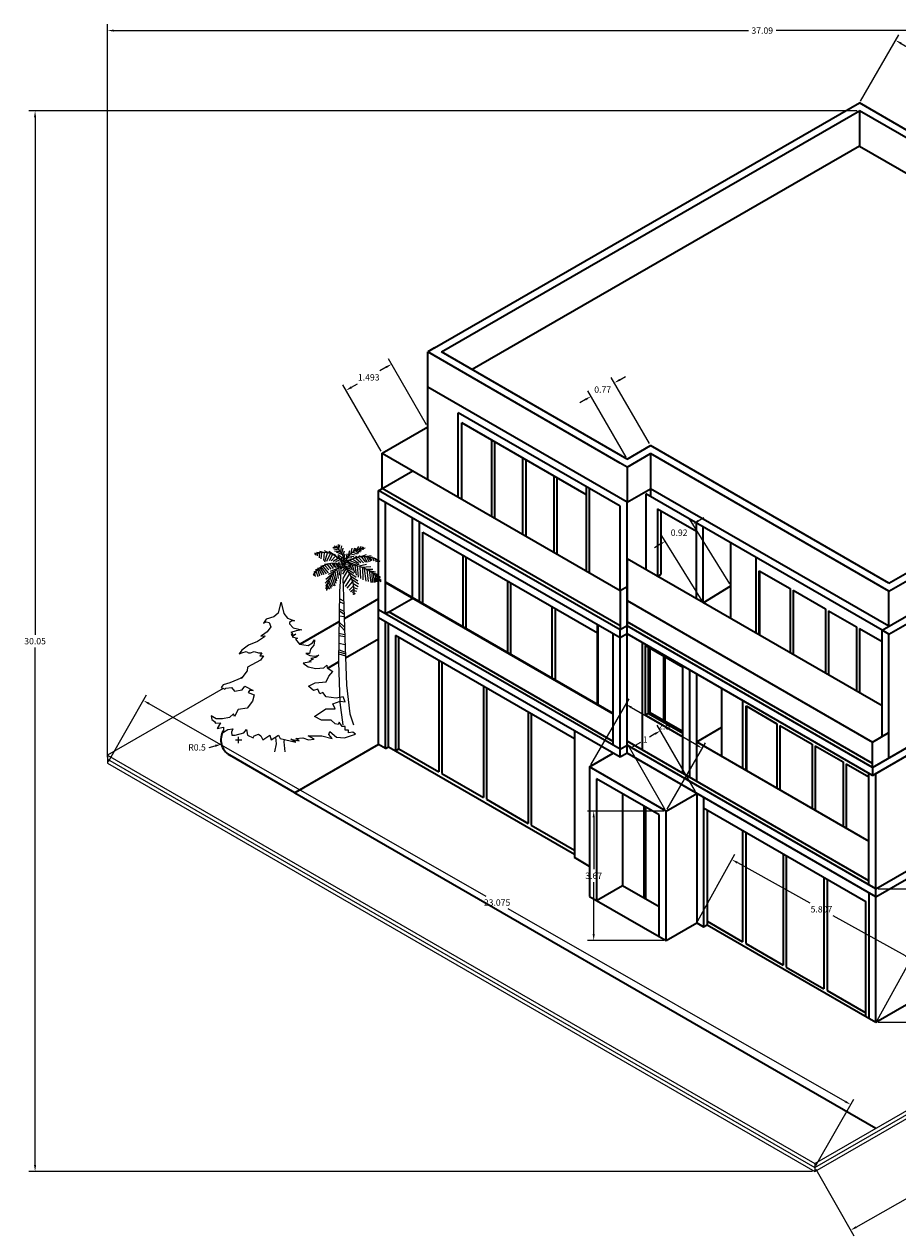
# Model space of a CAD drawing. Units: metres. Extents: x 5057 to 10150, y 1364 to 2760.
# Tile 1 of 2: x 5057 to 5082, y 1364 to 1399. Entities that reach past the tile are written whole.
import ezdxf

# ---------------------------------------------------------------- set-up
doc = ezdxf.new("R2010")
doc.units = ezdxf.units.M
for name, color, linetype, lineweight in [('A-ANNO-DIMS', 2, 'Continuous', 18), ('A-ANNO-NPLT', 8, 'Continuous', 13), ('A-ELEV', 7, 'Continuous', 35), ('C-SITE', 3, 'Continuous', 25), ('L-PLNT', 3, 'Continuous', 13)]:
    doc.layers.add(name, color=color, linetype=linetype, lineweight=lineweight)
doc.styles.get("Standard").update_dxf_attribs({"font": 'arial.ttf'})
doc.dimstyles.get("Standard").update_dxf_attribs({"dimtxt": 0.18, "dimasz": 0.18, "dimexe": 0.18, "dimexo": 0.0625, "dimgap": 0.09, "dimtad": 0, "dimtih": 1, "dimtoh": 1, "dimdec": 4, "dimzin": 0, "dimdsep": 46, "dimtxsty": 'Standard', "dimcen": 0.09, "dimadec": 0, "dimazin": 0, "dimtfac": 1, "dimtdec": 4, "dimtofl": 0, "dimtmove": 0, "dimatfit": 3, "dimfxl": 1, "dimtolj": 1, "dimtzin": 0, "dimarcsym": 0})

# ---------------------------------------------------------------- blocks, each defined once
blk = doc.blocks.new('*U3')
for p, q in [((-29.729, 190.759), (-31.469, 191.255)), ((-30.309, 190.512), (-30.695, 189.025)), ((-25.283, 191.751), (-29.342, 192.246)), ((-28.763, 190.759), (-28.763, 188.281)), ((-26.443, 191.503), (-26.636, 186.051)), ((-20.064, 191.751), (-25.863, 193.238)), ((-23.737, 191.751), (-24.51, 185.06)), ((-21.031, 191.998), (-21.804, 183.325)), ((-15.232, 191.255), (-20.644, 193.981)), ((-17.551, 191.503), (-20.451, 181.343)), ((-14.265, 190.759), (-18.131, 182.086)), ((-9.433, 189.025), (-15.618, 193.238)), ((-11.753, 189.768), (-15.425, 182.83)), ((-6.727, 197.202), (-11.366, 197.45)), ((-3.441, 194.477), (-10.013, 195.716)), ((-1.894, 192.494), (-9.24, 193.733)), ((-6.147, 186.299), (-9.24, 190.264)), ((-7.5, 199.68), (-7.5, 197.946)), ((-0.541, 189.52), (-7.307, 192.494)), ((-5.76, 190.016), (0.618, 185.308)), ((-5.567, 196.707), (-4.987, 201.167)), ((-4.407, 195.716), (-3.247, 200.672)), ((-2.474, 193.733), (-1.315, 199.433)), ((-1.121, 190.759), (0.232, 196.955)), ((0.038, 188.281), (1.778, 193.981)), ((1.005, 185.803), (2.358, 190.759)), ((4.098, 185.06), (4.678, 190.512)), ((5.837, 187.786), (7.577, 194.229)), ((8.544, 190.512), (13.763, 189.52)), ((9.317, 191.255), (10.283, 196.955)), ((11.25, 192.494), (15.889, 190.512)), ((11.829, 192.99), (13.182, 197.45)), ((13.956, 194.229), (14.729, 196.955)), ((14.536, 193.981), (17.242, 191.255)), ((15.116, 194.477), (17.822, 198.689)), ((16.082, 194.972), (17.822, 192.494)), ((18.015, 195.716), (20.914, 198.689)), ((18.015, 195.468), (18.981, 192.494)), ((19.368, 196.459), (19.948, 193.733)), ((19.368, 187.29), (26.133, 189.768)), ((20.914, 196.459), (21.301, 194.972)), ((21.301, 196.459), (22.847, 198.441)), ((22.074, 196.707), (23.427, 195.716)), ((23.234, 196.707), (23.62, 197.698)), ((-21.031, 177.626), (-24.897, 176.387)), ((-24.317, 175.891), (-18.711, 168.457)), ((-22.191, 176.635), (-16.391, 169.448)), ((-15.618, 179.36), (-20.644, 178.617)), ((-20.064, 177.626), (-15.812, 172.67)), ((-17.358, 178.617), (-13.299, 173.661)), ((-15.038, 179.36), (-10.786, 174.404)), ((-8.08, 188.034), (-12.912, 182.83)), ((-12.332, 180.104), (-9.433, 175.643)), ((-4.987, 185.803), (-10.979, 182.086)), ((-10.206, 180.104), (-8.08, 175.891)), ((-1.701, 176.882), (-8.66, 175.396)), ((-8.273, 180.104), (-6.147, 176.635)), ((-3.247, 183.821), (-8.08, 181.838)), ((-6.34, 179.608), (-4.6, 177.13)), ((-5.76, 188.034), (-1.508, 182.582)), ((-1.315, 181.591), (-5.374, 181.095)), ((-4.021, 179.36), (-2.861, 177.378)), ((-2.668, 185.803), (1.198, 181.343)), ((-2.668, 176.387), (-2.376, 170.594)), ((-0.348, 180.352), (-1.894, 180.104)), ((-0.928, 176.882), (-1.508, 173.909)), ((2.551, 175.891), (-0.928, 171.431)), ((1.585, 177.13), (0.038, 174.652)), ((1.005, 182.582), (2.938, 186.547)), ((1.585, 177.13), (6.61, 176.139)), ((2.938, 182.582), (6.61, 183.821)), ((2.938, 175.891), (8.737, 173.413)), ((4.098, 180.847), (8.35, 179.608)), ((4.871, 186.051), (10.09, 186.547)), ((4.871, 181.591), (8.544, 184.812)), ((5.644, 181.838), (13.569, 178.865)), ((6.224, 178.121), (8.157, 175.148)), ((6.997, 188.529), (12.216, 187.786)), ((7.384, 178.369), (10.476, 179.36)), ((7.77, 183.325), (16.082, 179.856)), ((8.157, 178.121), (10.476, 172.422)), ((9.51, 184.317), (15.502, 188.034)), ((10.476, 177.874), (12.796, 169.696)), ((11.25, 184.812), (17.628, 180.352)), ((11.829, 177.874), (18.015, 179.113)), ((13.182, 177.874), (14.729, 166.97)), ((14.536, 185.803), (19.948, 180.847)), ((15.695, 186.299), (19.368, 188.777)), ((15.889, 177.13), (16.855, 164.492)), ((17.242, 186.547), (23.041, 180.599)), ((18.015, 177.13), (26.133, 179.113)), ((18.981, 175.891), (19.561, 163.005)), ((20.721, 187.042), (25.167, 181.343)), ((20.914, 175.891), (30.966, 176.635)), ((23.814, 187.29), (26.907, 181.343)), ((24.78, 187.538), (31.546, 188.777)), ((26.133, 187.29), (29.419, 181.838)), ((28.066, 187.29), (30.966, 182.582)), ((29.806, 186.795), (32.319, 183.078)), ((29.999, 186.795), (33.092, 187.29)), ((32.512, 186.299), (35.218, 186.299)), ((33.479, 186.051), (34.445, 182.83)), ((35.605, 185.556), (37.151, 185.308)), ((35.798, 185.308), (36.958, 181.591)), ((38.118, 184.317), (38.504, 181.838)), ((39.857, 182.83), (40.244, 181.591)), ((-32.628, 167.961), (-33.208, 167.961)), ((-32.628, 167.713), (-32.435, 165.979)), ((-28.956, 172.174), (-32.435, 170.192)), ((-31.082, 169.944), (-32.435, 169.2)), ((-31.662, 168.705), (-31.082, 165.483)), ((-27.409, 173.413), (-30.695, 172.67)), ((-29.922, 170.687), (-27.989, 165.235)), ((-25.09, 175.148), (-28.376, 174.404)), ((-27.989, 172.422), (-26.056, 166.227)), ((-26.829, 173.661), (-23.544, 167.218)), ((-25.476, 174.652), (-21.224, 167.466)), ((-14.265, 164.244), (-19.678, 158.049)), ((-12.139, 167.961), (-19.098, 162.014)), ((-8.466, 171.678), (-16.585, 167.713)), ((-14.265, 163.749), (-10.786, 154.828)), ((-4.214, 175.148), (-14.072, 170.935)), ((-12.719, 166.722), (-9.046, 154.828)), ((-10.979, 168.457), (-7.887, 157.801)), ((-8.853, 170.935), (-7.113, 160.527)), ((-6.92, 172.917), (-5.374, 163.253)), ((-4.6, 174.9), (-4.021, 166.722)), ((3.711, 174.404), (-0.541, 167.961)), ((5.257, 171.926), (-0.155, 163.005)), ((7.384, 168.705), (0.812, 157.553)), ((9.317, 164.244), (2.358, 154.332)), ((4.291, 173.909), (12.216, 168.953)), ((6.417, 170.439), (14.729, 164.492)), ((8.544, 165.979), (16.662, 160.527)), ((10.09, 162.51), (17.435, 157.058)), ((21.688, 175.396), (22.074, 161.518)), ((23.814, 174.404), (25.554, 160.279)), ((25.554, 173.661), (33.285, 173.661)), ((26.52, 173.165), (28.066, 159.784)), ((28.839, 172.174), (36.378, 170.687)), ((29.226, 171.926), (30.966, 158.545)), ((30.966, 170.687), (38.891, 167.713)), ((32.126, 169.696), (32.512, 158.545)), ((34.058, 168.705), (34.445, 158.545)), ((35.412, 167.713), (41.404, 164.988)), ((36.378, 166.474), (35.605, 158.792)), ((37.731, 165.235), (36.958, 159.288)), ((37.924, 165.235), (41.404, 163.749)), ((38.504, 164.492), (38.504, 159.536)), ((39.664, 163.253), (42.37, 161.766)), ((39.857, 162.757), (39.857, 160.031)), ((-16.005, 160.031), (-19.484, 154.084)), ((-18.131, 153.589), (-19.484, 151.606)), ((-17.938, 152.597), (-16.972, 151.111)), ((-17.358, 155.819), (-14.845, 151.358)), ((-16.585, 158.545), (-13.106, 152.35)), ((-15.618, 160.775), (-12.332, 154.332)), ((10.863, 159.784), (4.484, 152.35)), ((11.829, 155.075), (6.804, 150.119)), ((12.603, 151.111), (8.544, 148.385)), ((11.443, 157.553), (16.855, 154.332)), ((12.216, 153.093), (16.082, 151.606)), ((12.603, 149.872), (15.116, 149.128)), ((40.824, 161.766), (41.21, 160.031)), ((41.21, 161.518), (42.757, 160.279)), ((-4.081, 140.645), (0.753, 138.261)), ((-4.081, 137.547), (0.753, 135.163)), ((12.216, 148.137), (10.09, 147.393)), ((12.409, 145.659), (11.056, 145.659)), ((12.409, 146.898), (13.763, 146.402)), ((-4.081, 129.205), (1.124, 126.821)), ((-4.081, 127.298), (1.31, 123.246)), ((-4.453, 112.283), (1.682, 105.133)), ((-4.267, 114.428), (1.682, 108.708)), ((-4.081, 121.578), (1.31, 120.863)), ((-4.639, 102.273), (1.868, 100.604)), ((-4.453, 99.651), (2.24, 98.459)), ((-4.825, 83.921), (2.612, 81.061)), ((-4.639, 81.299), (2.797, 78.916)), ((-4.453, 91.071), (2.426, 89.641)), ((-4.639, 78.916), (2.797, 76.771))]:
    blk.add_line(p, q)
for points in [[(-2.363, 170.553), (-3.88, 148.505), (-4.988, 69.634), (-3.325, 24.869), (0, 0)], [(-0.116, 162.848), (0.554, 143.532), (2.217, 96.635), (3.88, 44.054), (7.76, 12.079), (11.64, 0)]]:
    blk.add_lwpolyline(points)
for centre, radius, start, end in [((-21.738, 166.094), 25.899, 27.67115, 112.5305), ((-18.427, 181.448), 19.715, 350.285, 64.11229), ((25.595, 171.567), 25.395, 91.40319, 163.882), ((-9.259, 151.732), 28.386, 68.38311, 147.5322), ((14.394, 148.393), 32.752, 113.7592, 177.4133), ((23.687, 155.341), 32.188, 56.19272, 134.3213), ((5.828, 132.718), 45.639, 35.98777, 95.82273), ((-32.8, 147.923), 45.309, 356.1943, 41.37848)]:
    blk.add_arc(centre, radius, start, end)
blk = doc.blocks.new('*U5')
for p, q in [((-8.263, 7.598), (-8.747, 14.105)), ((-0.771, 9.56), (-0.69, 11.833)), ((-9.75, 0), (-8.263, 7.598)), ((0, 0), (-0.771, 9.56))]:
    blk.add_line(p, q)
for points in [[(-3.9, 142.35), (-6.596, 132.037), (-10.801, 128.443), (-17.81, 126.047), (-20.614, 122.452), (-17.81, 123.65), (-15.007, 123.051), (-13.605, 118.858), (-16.876, 114.065), (-21.549, 111.07), (-22.951, 109.872), (-19.212, 110.471), (-19.68, 109.273), (-26.222, 105.079), (-34.633, 101.485), (-41.175, 96.693), (-43.511, 93.098), (-41.175, 94.296), (-36.969, 95.494), (-34.633, 94.296), (-32.764, 94.296), (-29.493, 95.494)], [(-3.759, 141.97), (-1.074, 131.643), (2.437, 127.141), (8.84, 124.493), (6.568, 124.493), (4.09, 123.169), (4.296, 121.846), (7.807, 117.874), (16.069, 116.02), (10.492, 115.226), (5.535, 113.372), (6.981, 112.843), (5.948, 110.989), (10.286, 112.048), (6.775, 109.401), (11.732, 108.077), (9.873, 107.282), (13.797, 102.516), (21.852, 101.192), (25.983, 103.84), (28.048, 106.488), (27.842, 105.164), (27.429, 101.457), (24.124, 97.75), (23.091, 93.513), (19.58, 93.513), (23.505, 91.66), (28.255, 90.866), (31.973, 91.925), (29.081, 89.806), (24.537, 88.747), (26.809, 88.218), (22.472, 86.099), (24.95, 85.57), (17.308, 84.246), (21.852, 80.804), (29.081, 79.215), (36.723, 80.009), (39.821, 82.392), (40.028, 80.009), (45.398, 76.567)], [(-29.25, 95.55), (-25.287, 94.296), (-22.016, 94.296), (-23.885, 91.301), (-20.614, 91.301), (-23.418, 87.108), (-35.567, 80.518), (-36.035, 76.924), (-41.175, 70.334), (-52.389, 65.542), (-58.931, 63.744), (-60.8, 61.348), (-57.062, 59.551), (-56.128, 60.749), (-50.987, 61.348), (-48.184, 57.754), (-40.707, 58.952), (-38.371, 62.546), (-30.427, 58.353), (-33.698, 58.353), (-35.1, 56.556), (-29.493, 54.159), (-30.894, 48.169), (-36.035, 41.579), (-44.446, 40.381), (-48.184, 33.791), (-49.118, 36.188), (-52.857, 32.593), (-59.399, 31.395), (-65.473, 31.395), (-70.146, 34.39), (-69.679, 30.796), (-66.875, 28.999), (-65.941, 27.202), (-61.268, 27.801), (-64.539, 22.409), (-58.464, 23.607), (-58.464, 18.815), (-54.258, 21.211), (-49.586, 21.81), (-50.987, 18.815), (-50.52, 15.82), (-47.249, 15.82), (-39.306, 18.216), (-36.502, 21.211), (-35.567, 15.82), (-30.427, 13.423), (-29.493, 15.221), (-25.287, 17.018), (-22.951, 15.221), (-21.081, 11.626), (-14.539, 15.82), (-13.138, 11.626), (-6.128, 15.82), (-4.726, 12.824), (10.226, 9.23), (5.554, 12.225), (13.497, 10.428), (10.226, 12.824), (16.768, 13.423), (22.376, 11.626), (27.516, 12.225), (21.909, 15.221), (34.993, 15.221), (44.806, 12.824), (41.535, 16.419), (42.469, 19.414), (49.011, 14.023), (56.487, 13.423), (66.768, 17.018), (64.431, 18.815), (60.226, 18.216), (60.226, 20.612), (56.955, 20.612), (56.955, 24.206), (54.151, 24.206), (51.348, 28.4), (50.413, 26.004), (47.609, 26.603), (43.871, 30.197), (38.731, 30.197), (34.525, 30.197), (27.983, 33.791), (38.731, 40.98), (47.609, 40.98), (45.273, 45.773), (52.282, 48.169), (56.955, 47.57), (55.086, 52.362), (48.544, 51.164), (39.198, 52.362), (35.927, 56.556), (33.123, 55.357), (31.254, 59.551), (27.049, 58.353), (22.376, 62.546), (28.451, 65.542), (39.198, 66.74), (41.535, 72.131), (45.273, 76.325)]]:
    blk.add_lwpolyline(points)
blk = doc.blocks.new('*D9')
at = {"layer": 'A-ANNO-DIMS', "color": 0, "lineweight": -2, "transparency": 16777216}
for p, q in [((5059.194, 1377.756), (5059.194, 1398.523)), ((5059.374, 1398.343), (5077.345, 1398.343)), ((5096.103, 1398.343), (5078.132, 1398.343)), ((5096.283, 1375.925), (5096.283, 1398.523))]:
    blk.add_line(p, q, dxfattribs=at)
at = {"layer": 'A-ANNO-DIMS', "color": 0, "transparency": 16777216}
for points in [[(5059.374, 1398.373), (5059.374, 1398.313), (5059.194, 1398.343)], [(5096.103, 1398.373), (5096.103, 1398.313), (5096.283, 1398.343)]]:
    blk.add_solid(points, dxfattribs=at)
at = {"layer": 'Defpoints', "color": 0, "transparency": 16777216}
for p in [(5096.283, 1398.343), (5059.194, 1377.694), (5096.283, 1375.863)]:
    blk.add_point(p, dxfattribs=at)
at = {"layer": 'A-ANNO-DIMS', "color": 0, "transparency": 16777216, "insert": (5077.738, 1398.343), "char_height": 0.18, "attachment_point": 5}
blk.add_mtext('\\A1;37.09', dxfattribs=at)
blk = doc.blocks.new('*D10')
at = {"layer": 'A-ANNO-DIMS', "color": 0, "lineweight": -2, "transparency": 16777216}
for p, q in [((5080.427, 1396.067), (5056.964, 1396.067)), ((5057.144, 1395.887), (5057.144, 1381.223)), ((5057.144, 1366.195), (5057.144, 1380.859)), ((5079.164, 1366.015), (5056.964, 1366.015))]:
    blk.add_line(p, q, dxfattribs=at)
at = {"layer": 'A-ANNO-DIMS', "color": 0, "transparency": 16777216}
for points in [[(5057.114, 1395.887), (5057.174, 1395.887), (5057.144, 1396.067)], [(5057.114, 1366.195), (5057.174, 1366.195), (5057.144, 1366.015)]]:
    blk.add_solid(points, dxfattribs=at)
at = {"layer": 'Defpoints', "color": 0, "transparency": 16777216}
for p in [(5057.144, 1396.067), (5080.489, 1396.067), (5079.226, 1366.015)]:
    blk.add_point(p, dxfattribs=at)
at = {"layer": 'A-ANNO-DIMS', "color": 0, "transparency": 16777216, "insert": (5057.144, 1381.041), "char_height": 0.18, "attachment_point": 5}
blk.add_mtext('\\A1;30.05', dxfattribs=at)
blk = doc.blocks.new('*D11')
at = {"layer": 'A-ANNO-DIMS', "color": 0, "lineweight": -2, "transparency": 16777216}
for p, q in [((5059.225, 1377.635), (5060.301, 1379.517)), ((5060.368, 1379.271), (5069.909, 1373.816)), ((5080.088, 1367.997), (5070.546, 1373.452)), ((5079.257, 1366.182), (5080.333, 1368.064))]:
    blk.add_line(p, q, dxfattribs=at)
at = {"layer": 'A-ANNO-DIMS', "color": 0, "transparency": 16777216}
for points in [[(5060.383, 1379.297), (5060.353, 1379.245), (5060.211, 1379.36)], [(5080.102, 1368.023), (5080.073, 1367.971), (5080.244, 1367.908)]]:
    blk.add_solid(points, dxfattribs=at)
at = {"layer": 'Defpoints', "color": 0, "transparency": 16777216}
for p in [(5059.194, 1377.581), (5080.244, 1367.908), (5079.226, 1366.128)]:
    blk.add_point(p, dxfattribs=at)
at = {"layer": 'A-ANNO-DIMS', "color": 0, "transparency": 16777216, "insert": (5070.228, 1373.634), "char_height": 0.18, "attachment_point": 5}
blk.add_mtext('\\A1;23.075', dxfattribs=at)
blk = doc.blocks.new('*D12')
at = {"layer": 'A-ANNO-DIMS', "color": 0, "lineweight": -2, "transparency": 16777216}
for p, q in [((5096.314, 1375.808), (5097.388, 1373.926)), ((5097.143, 1373.993), (5089.09, 1369.397)), ((5080.399, 1364.437), (5088.452, 1369.033)), ((5079.257, 1366.074), (5080.332, 1364.191))]:
    blk.add_line(p, q, dxfattribs=at)
at = {"layer": 'A-ANNO-DIMS', "color": 0, "transparency": 16777216}
for points in [[(5097.128, 1374.019), (5097.158, 1373.967), (5097.299, 1374.082)], [(5080.384, 1364.463), (5080.414, 1364.411), (5080.243, 1364.348)]]:
    blk.add_solid(points, dxfattribs=at)
at = {"layer": 'Defpoints', "color": 0, "transparency": 16777216}
for p in [(5096.283, 1375.863), (5079.226, 1366.128), (5080.243, 1364.348)]:
    blk.add_point(p, dxfattribs=at)
at = {"layer": 'A-ANNO-DIMS', "color": 0, "transparency": 16777216, "insert": (5088.771, 1369.215), "char_height": 0.18, "attachment_point": 5}
blk.add_mtext('\\A1;19.64', dxfattribs=at)
blk = doc.blocks.new('*D17')
at = {"layer": 'A-ANNO-DIMS', "color": 0, "lineweight": -2, "transparency": 16777216}
for p, q in [((5080.521, 1396.347), (5081.604, 1398.224)), ((5081.67, 1397.979), (5084.681, 1396.24)), ((5088.323, 1394.138), (5085.312, 1395.876)), ((5087.485, 1392.327), (5088.569, 1394.204))]:
    blk.add_line(p, q, dxfattribs=at)
at = {"layer": 'A-ANNO-DIMS', "color": 0, "transparency": 16777216}
for points in [[(5081.685, 1398.005), (5081.655, 1397.953), (5081.514, 1398.069)], [(5088.338, 1394.164), (5088.308, 1394.112), (5088.479, 1394.048)]]:
    blk.add_solid(points, dxfattribs=at)
at = {"layer": 'Defpoints', "color": 0, "transparency": 16777216}
for p in [(5080.489, 1396.293), (5088.479, 1394.048), (5087.454, 1392.272)]:
    blk.add_point(p, dxfattribs=at)
at = {"layer": 'A-ANNO-DIMS', "color": 0, "transparency": 16777216, "insert": (5084.997, 1396.058), "char_height": 0.18, "attachment_point": 5}
blk.add_mtext('\\A1;8.042', dxfattribs=at)
blk = doc.blocks.new('*D24')
at = {"layer": 'A-ANNO-DIMS', "color": 0, "lineweight": -2, "transparency": 16777216}
for p, q in [((5072.881, 1377.532), (5073.965, 1379.409)), ((5074.031, 1379.163), (5074.701, 1378.776)), ((5075.884, 1378.093), (5075.213, 1378.48)), ((5075.046, 1376.282), (5076.13, 1378.159))]:
    blk.add_line(p, q, dxfattribs=at)
at = {"layer": 'A-ANNO-DIMS', "color": 0, "transparency": 16777216}
for points in [[(5074.046, 1379.189), (5074.016, 1379.137), (5073.875, 1379.253)], [(5075.899, 1378.119), (5075.869, 1378.067), (5076.04, 1378.003)]]:
    blk.add_solid(points, dxfattribs=at)
at = {"layer": 'Defpoints', "color": 0, "transparency": 16777216}
for p in [(5076.04, 1378.003), (5072.85, 1377.478), (5075.015, 1376.228)]:
    blk.add_point(p, dxfattribs=at)
at = {"layer": 'A-ANNO-DIMS', "color": 0, "transparency": 16777216, "insert": (5074.957, 1378.628), "char_height": 0.18, "attachment_point": 5}
blk.add_mtext('\\A1;2.5', dxfattribs=at)
blk = doc.blocks.new('*D25')
at = {"layer": 'A-ANNO-DIMS', "color": 0, "lineweight": -2, "transparency": 16777216}
for p, q in [((5075.85, 1376.782), (5074.766, 1378.659)), ((5074.984, 1376.282), (5073.9, 1378.159)), ((5074.146, 1378.093), (5074.3, 1378.182)), ((5074.7, 1378.413), (5074.546, 1378.324))]:
    blk.add_line(p, q, dxfattribs=at)
at = {"layer": 'A-ANNO-DIMS', "color": 0, "transparency": 16777216}
for points in [[(5074.685, 1378.439), (5074.715, 1378.387), (5074.856, 1378.503)], [(5074.131, 1378.119), (5074.161, 1378.067), (5073.99, 1378.003)]]:
    blk.add_solid(points, dxfattribs=at)
at = {"layer": 'Defpoints', "color": 0, "transparency": 16777216}
for p in [(5074.856, 1378.503), (5075.881, 1376.728), (5075.015, 1376.228)]:
    blk.add_point(p, dxfattribs=at)
at = {"layer": 'A-ANNO-DIMS', "color": 0, "transparency": 16777216, "insert": (5074.423, 1378.253), "char_height": 0.18, "attachment_point": 5}
blk.add_mtext('\\A1;1', dxfattribs=at)
blk = doc.blocks.new('*D26')
at = {"layer": 'A-ANNO-DIMS', "color": 0, "lineweight": -2, "transparency": 16777216}
for p, q in [((5074.952, 1376.228), (5072.785, 1376.228)), ((5072.965, 1376.048), (5072.965, 1374.576)), ((5072.965, 1372.74), (5072.965, 1374.212)), ((5074.952, 1372.56), (5072.785, 1372.56))]:
    blk.add_line(p, q, dxfattribs=at)
at = {"layer": 'A-ANNO-DIMS', "color": 0, "transparency": 16777216}
for points in [[(5072.935, 1376.048), (5072.995, 1376.048), (5072.965, 1376.228)], [(5072.935, 1372.74), (5072.995, 1372.74), (5072.965, 1372.56)]]:
    blk.add_solid(points, dxfattribs=at)
at = {"layer": 'Defpoints', "color": 0, "transparency": 16777216}
for p in [(5072.965, 1376.228), (5075.015, 1376.228), (5075.015, 1372.56)]:
    blk.add_point(p, dxfattribs=at)
at = {"layer": 'A-ANNO-DIMS', "color": 0, "transparency": 16777216, "insert": (5072.965, 1374.394), "char_height": 0.18, "attachment_point": 5}
blk.add_mtext('\\A1;3.67', dxfattribs=at)
blk = doc.blocks.new('*D27')
at = {"layer": 'A-ANNO-DIMS', "color": 0, "lineweight": -2, "transparency": 16777216}
for p, q in [((5075.911, 1373.114), (5076.963, 1375.009)), ((5077.033, 1374.765), (5079.087, 1373.625)), ((5081.796, 1372.121), (5079.742, 1373.261)), ((5080.989, 1370.296), (5082.041, 1372.191))]:
    blk.add_line(p, q, dxfattribs=at)
at = {"layer": 'A-ANNO-DIMS', "color": 0, "transparency": 16777216}
for points in [[(5077.048, 1374.791), (5077.019, 1374.738), (5076.876, 1374.852)], [(5081.811, 1372.147), (5081.781, 1372.095), (5081.953, 1372.033)]]:
    blk.add_solid(points, dxfattribs=at)
at = {"layer": 'Defpoints', "color": 0, "transparency": 16777216}
for p in [(5075.881, 1373.06), (5081.953, 1372.033), (5080.958, 1370.241)]:
    blk.add_point(p, dxfattribs=at)
at = {"layer": 'A-ANNO-DIMS', "color": 0, "transparency": 16777216, "insert": (5079.415, 1373.443), "char_height": 0.18, "attachment_point": 5}
blk.add_mtext('\\A1;5.807', dxfattribs=at)
blk = doc.blocks.new('*D28')
at = {"layer": 'A-ANNO-DIMS', "color": 0, "lineweight": -2, "transparency": 16777216}
for p, q in [((5081.021, 1374.022), (5098.513, 1374.022)), ((5098.333, 1373.842), (5098.333, 1372.314)), ((5098.333, 1370.421), (5098.333, 1371.95)), ((5081.021, 1370.241), (5098.513, 1370.241))]:
    blk.add_line(p, q, dxfattribs=at)
at = {"layer": 'A-ANNO-DIMS', "color": 0, "transparency": 16777216}
for points in [[(5098.303, 1373.842), (5098.363, 1373.842), (5098.333, 1374.022)], [(5098.303, 1370.421), (5098.363, 1370.421), (5098.333, 1370.241)]]:
    blk.add_solid(points, dxfattribs=at)
at = {"layer": 'Defpoints', "color": 0, "transparency": 16777216}
for p in [(5080.958, 1374.022), (5098.333, 1374.022), (5080.958, 1370.241)]:
    blk.add_point(p, dxfattribs=at)
at = {"layer": 'A-ANNO-DIMS', "color": 0, "transparency": 16777216, "insert": (5098.333, 1372.132), "char_height": 0.18, "attachment_point": 5}
blk.add_mtext('\\A1;3.78', dxfattribs=at)
blk = doc.blocks.new('*D29')
at = {"layer": 'A-ANNO-DIMS', "color": 0, "lineweight": -2, "transparency": 16777216}
for p, q in [((5067.084, 1388.801), (5066.909, 1388.699)), ((5068.234, 1387.169), (5067.15, 1389.046)), ((5066.941, 1386.423), (5065.857, 1388.3)), ((5066.103, 1388.234), (5066.278, 1388.335))]:
    blk.add_line(p, q, dxfattribs=at)
at = {"layer": 'A-ANNO-DIMS', "color": 0, "transparency": 16777216}
for points in [[(5067.069, 1388.827), (5067.099, 1388.775), (5067.24, 1388.891)], [(5066.088, 1388.26), (5066.118, 1388.208), (5065.947, 1388.144)]]:
    blk.add_solid(points, dxfattribs=at)
at = {"layer": 'Defpoints', "color": 0, "transparency": 16777216}
for p in [(5067.24, 1388.891), (5068.265, 1387.115), (5066.972, 1386.369)]:
    blk.add_point(p, dxfattribs=at)
at = {"layer": 'A-ANNO-DIMS', "color": 0, "transparency": 16777216, "insert": (5066.593, 1388.517), "char_height": 0.18, "attachment_point": 5}
blk.add_mtext('\\A1;1.493', dxfattribs=at)
blk = doc.blocks.new('*D30')
at = {"layer": 'A-ANNO-DIMS', "color": 0, "lineweight": -2, "transparency": 16777216}
for p, q in [((5074.545, 1386.639), (5073.461, 1388.516)), ((5073.707, 1388.45), (5073.863, 1388.54)), ((5073.88, 1386.255), (5072.797, 1388.132)), ((5072.731, 1387.887), (5072.575, 1387.797))]:
    blk.add_line(p, q, dxfattribs=at)
at = {"layer": 'A-ANNO-DIMS', "color": 0, "transparency": 16777216}
for points in [[(5073.692, 1388.476), (5073.722, 1388.424), (5073.551, 1388.36)], [(5072.716, 1387.913), (5072.746, 1387.861), (5072.887, 1387.977)]]:
    blk.add_solid(points, dxfattribs=at)
at = {"layer": 'Defpoints', "color": 0, "transparency": 16777216}
for p in [(5073.551, 1388.36), (5074.576, 1386.585), (5073.912, 1386.201)]:
    blk.add_point(p, dxfattribs=at)
at = {"layer": 'A-ANNO-DIMS', "color": 0, "transparency": 16777216, "insert": (5073.219, 1388.168), "char_height": 0.18, "attachment_point": 5}
blk.add_mtext('\\A1;0.77', dxfattribs=at)
blk = doc.blocks.new('*D31')
at = {"layer": 'A-ANNO-DIMS', "color": 0, "lineweight": -2, "transparency": 16777216}
for p, q in [((5076.816, 1382.663), (5075.68, 1384.509)), ((5075.928, 1384.45), (5076.081, 1384.544)), ((5076.035, 1382.182), (5074.898, 1384.028)), ((5074.84, 1383.78), (5074.686, 1383.686))]:
    blk.add_line(p, q, dxfattribs=at)
at = {"layer": 'A-ANNO-DIMS', "color": 0, "transparency": 16777216}
for points in [[(5075.912, 1384.475), (5075.943, 1384.424), (5075.774, 1384.356)], [(5074.824, 1383.806), (5074.855, 1383.754), (5074.993, 1383.874)]]:
    blk.add_solid(points, dxfattribs=at)
at = {"layer": 'Defpoints', "color": 0, "transparency": 16777216}
for p in [(5075.774, 1384.356), (5076.849, 1382.61), (5076.067, 1382.129)]:
    blk.add_point(p, dxfattribs=at)
at = {"layer": 'A-ANNO-DIMS', "color": 0, "transparency": 16777216, "insert": (5075.384, 1384.115), "char_height": 0.18, "attachment_point": 5}
blk.add_mtext('\\A1;0.92', dxfattribs=at)
blk = doc.blocks.new('*D32')
at = {"layer": 'A-ANNO-DIMS', "color": 0, "lineweight": -2, "transparency": 16777216}
for p, q in [((5062.816, 1378.241), (5062.996, 1378.241)), ((5062.906, 1378.151), (5062.906, 1378.331)), ((5062.072, 1378.031), (5062.246, 1378.075))]:
    blk.add_line(p, q, dxfattribs=at)
at = {"layer": 'A-ANNO-DIMS', "color": 0, "transparency": 16777216}
blk.add_solid([(5062.239, 1378.104), (5062.254, 1378.046), (5062.421, 1378.119)], dxfattribs=at)
at = {"layer": 'Defpoints', "color": 0, "transparency": 16777216}
for p in [(5062.421, 1378.119), (5062.906, 1378.241)]:
    blk.add_point(p, dxfattribs=at)
at = {"layer": 'A-ANNO-DIMS', "color": 0, "transparency": 16777216, "insert": (5061.731, 1378.031), "char_height": 0.18, "attachment_point": 5}
blk.add_mtext('\\A1;R0.5', dxfattribs=at)

msp = doc.modelspace()

# ---------------------------------------------------------------- linework, layer by layer
at = {"layer": 'A-ANNO-NPLT'}
for p in [(5069.2979, 1383.4577), (5070.5622, 1382.7278), (5071.8265, 1381.9978), (5068.6184, 1380.4689), (5069.8845, 1379.7379), (5071.1507, 1379.0069), (5077.2265, 1375.651), (5078.3764, 1374.9872), (5079.5263, 1374.3233)]:
    msp.add_point(p, dxfattribs=at)
at = {"layer": 'A-ELEV'}
for p, q in [((5068.4606, 1389.3484), (5080.4894, 1396.2932)), ((5087.4536, 1392.2724), (5080.4894, 1396.2932)), ((5068.6563, 1389.2354), (5080.4894, 1396.0672)), ((5087.0622, 1392.2724), (5080.4894, 1396.0672)), ((5080.4894, 1396.0672), (5080.4894, 1395.0672)), ((5080.4894, 1395.0672), (5069.5224, 1388.7354)), ((5080.4894, 1395.0672), (5086.1962, 1391.7724)), ((5068.4606, 1389.3484), (5068.2649, 1389.2354)), ((5073.7159, 1386.0882), (5068.2649, 1389.2354)), ((5068.2649, 1388.2354), (5068.2649, 1389.2354)), ((5073.9116, 1386.2012), (5068.6563, 1389.2354)), ((5081.3272, 1382.4613), (5092.8871, 1389.1354)), ((5081.3272, 1382.6873), (5092.4956, 1389.1354)), ((5073.9116, 1384.9752), (5068.2649, 1388.2354)), ((5068.2649, 1385.6224), (5068.2649, 1388.2354)), ((5081.1315, 1381.3483), (5092.8871, 1388.1354)), ((5081.3272, 1381.2353), (5093.0828, 1388.0224)), ((5073.7159, 1384.8622), (5069.1309, 1387.5094)), ((5069.1309, 1385.1224), (5069.1309, 1387.5094)), ((5066.972, 1386.3688), (5068.2649, 1387.1152)), ((5072.7633, 1385.1862), (5069.2288, 1387.2269)), ((5069.2288, 1385.0659), (5069.2288, 1387.2269)), ((5070.0691, 1386.7417), (5070.0691, 1384.5807)), ((5070.1557, 1386.6917), (5070.1557, 1384.5307)), ((5066.972, 1385.3688), (5066.972, 1386.3688)), ((5066.972, 1386.3688), (5073.7159, 1382.4752)), ((5073.9116, 1386.2012), (5074.5762, 1386.585)), ((5073.9116, 1385.9752), (5074.5762, 1386.359)), ((5081.3272, 1382.6873), (5074.5762, 1386.585)), ((5081.3272, 1382.4613), (5074.5762, 1386.359)), ((5074.5762, 1386.359), (5074.5762, 1385.133)), ((5070.9527, 1386.2316), (5070.9527, 1384.0706)), ((5071.0393, 1386.1816), (5071.0393, 1384.0206)), ((5073.9116, 1385.9752), (5073.7159, 1386.0882)), ((5066.9231, 1385.3406), (5067.8381, 1385.8688)), ((5071.8363, 1385.7214), (5071.8363, 1383.5604)), ((5071.9229, 1385.6714), (5071.9229, 1383.5104)), ((5073.9116, 1385.9752), (5073.9116, 1384.9752)), ((5066.8742, 1385.3123), (5066.972, 1385.3688)), ((5066.8742, 1381.928), (5066.8742, 1385.3123)), ((5073.7159, 1381.3622), (5066.8742, 1385.3123)), ((5073.7159, 1381.4752), (5066.972, 1385.3688)), ((5072.7633, 1383.0252), (5072.7633, 1385.4122)), ((5072.8499, 1382.9752), (5072.8499, 1385.3622)), ((5073.9116, 1384.9752), (5074.5762, 1385.359)), ((5081.3272, 1381.4613), (5074.5762, 1385.359)), ((5073.7159, 1381.1362), (5066.8742, 1385.0863)), ((5067.0699, 1381.815), (5067.0699, 1384.9733)), ((5073.9116, 1381.4752), (5073.9116, 1384.9752)), ((5081.1315, 1381.3483), (5074.4391, 1385.2121)), ((5074.4391, 1385.2121), (5074.4391, 1383.0688)), ((5073.7159, 1382.4752), (5073.7159, 1384.8622)), ((5074.7719, 1384.794), (5075.8717, 1384.159)), ((5074.7719, 1384.794), (5074.7719, 1382.8766)), ((5074.8698, 1384.7375), (5074.8698, 1382.9331)), ((5067.8341, 1382.2562), (5067.8341, 1384.5321)), ((5068.0298, 1382.1632), (5068.0298, 1384.4191)), ((5075.8717, 1382.2416), (5075.8717, 1384.385)), ((5076.0675, 1382.1286), (5076.0675, 1384.272)), ((5080.8583, 1377.4646), (5093.0828, 1384.5224)), ((5080.8583, 1377.2386), (5093.0828, 1384.2964)), ((5068.1277, 1384.1333), (5073.0698, 1381.28)), ((5068.1277, 1382.1067), (5068.1277, 1384.1333)), ((5076.8491, 1381.6774), (5076.8491, 1383.8207)), ((5069.2546, 1383.4827), (5069.2546, 1381.4561)), ((5069.3412, 1383.4327), (5069.3412, 1381.4061)), ((5073.9116, 1378.0909), (5073.9116, 1383.3733)), ((5081.1315, 1379.2049), (5073.9116, 1383.3733)), ((5073.9116, 1383.3733), (5073.9116, 1381.4752)), ((5077.5689, 1381.2618), (5077.5689, 1383.4051)), ((5074.7719, 1382.8766), (5074.8698, 1382.9331)), ((5077.6555, 1383.0356), (5078.5255, 1382.5333)), ((5077.6555, 1381.2118), (5077.6555, 1383.0356)), ((5077.6728, 1381.2018), (5077.6728, 1383.0256)), ((5067.0872, 1382.7074), (5067.0699, 1382.6974)), ((5073.5202, 1378.9733), (5067.0699, 1382.6974)), ((5073.5202, 1378.9933), (5067.0872, 1382.7074)), ((5070.5189, 1382.7528), (5070.5189, 1380.7261)), ((5070.6055, 1382.7028), (5070.6055, 1380.6761)), ((5073.7159, 1382.4752), (5073.9116, 1382.5882)), ((5076.0675, 1382.1286), (5076.8491, 1382.6098)), ((5066.8742, 1382.2409), (5065.8987, 1381.6777)), ((5067.0699, 1381.815), (5067.8588, 1382.2704)), ((5073.7159, 1382.4752), (5073.7159, 1381.3622)), ((5078.5255, 1382.5333), (5078.5255, 1380.7095)), ((5078.6121, 1382.4833), (5078.6121, 1380.6595)), ((5078.6121, 1382.4833), (5079.526, 1381.9557)), ((5081.3272, 1381.4613), (5081.3272, 1382.4613)), ((5073.7159, 1377.9779), (5066.8742, 1381.928)), ((5066.8742, 1378.1094), (5066.8742, 1381.928)), ((5067.0699, 1381.815), (5067.1638, 1381.8692)), ((5073.5202, 1378.1993), (5067.1638, 1381.8692)), ((5071.7832, 1382.0228), (5071.7832, 1379.9961)), ((5071.8698, 1381.9728), (5071.8698, 1379.9461)), ((5073.9116, 1382.1933), (5080.8583, 1378.1826)), ((5079.526, 1381.9557), (5079.526, 1380.1318)), ((5079.6161, 1381.9037), (5079.6161, 1380.0799)), ((5079.6161, 1381.9037), (5080.4051, 1381.4481)), ((5065.7513, 1381.5926), (5064.6491, 1380.9562)), ((5073.7159, 1377.7519), (5066.8742, 1381.702)), ((5067.0699, 1377.9964), (5067.0699, 1381.589)), ((5067.1565, 1378.0464), (5067.1565, 1381.539)), ((5080.8583, 1377.5776), (5073.9116, 1381.5882)), ((5067.3522, 1381.2), (5067.3522, 1377.9334)), ((5072.4168, 1378.2759), (5067.3522, 1381.2)), ((5073.0698, 1379.2533), (5073.0698, 1381.5092)), ((5073.0871, 1379.2433), (5073.0871, 1381.4992)), ((5073.5202, 1378.0909), (5073.5202, 1381.2492)), ((5073.5202, 1379.1993), (5073.5202, 1381.2492)), ((5073.9116, 1381.4752), (5073.7159, 1381.3622)), ((5073.7159, 1377.9779), (5073.7159, 1381.3622)), ((5073.9116, 1381.2492), (5073.7159, 1381.1362)), ((5080.8583, 1377.4646), (5073.9116, 1381.4752)), ((5080.8583, 1377.2386), (5073.9116, 1381.2492)), ((5080.4051, 1381.4481), (5080.4051, 1379.6243)), ((5080.4901, 1381.3991), (5080.4901, 1379.5752)), ((5080.4901, 1381.3991), (5081.1315, 1381.0288)), ((5081.1315, 1378.3403), (5081.1315, 1381.3483)), ((5081.3272, 1381.2353), (5081.1315, 1381.3483)), ((5081.3272, 1377.7353), (5081.3272, 1381.2353)), ((5065.9359, 1380.5677), (5066.8742, 1381.1094)), ((5067.4501, 1377.9899), (5067.4501, 1381.1435)), ((5074.3446, 1377.9539), (5074.3446, 1380.9992)), ((5074.4312, 1378.9453), (5074.4312, 1380.9149)), ((5074.4312, 1380.9149), (5075.4895, 1380.3039)), ((5074.5178, 1378.9953), (5074.5178, 1380.8649)), ((5074.5659, 1379.023), (5074.5659, 1380.8371)), ((5080.9585, 1374.0224), (5093.0828, 1381.0224)), ((5068.5751, 1380.4939), (5068.5751, 1377.3404)), ((5074.9387, 1380.6219), (5074.9387, 1378.8078)), ((5074.982, 1380.5969), (5074.982, 1378.7828)), ((5065.433, 1380.2774), (5065.7353, 1380.4519)), ((5068.6617, 1380.4439), (5068.6617, 1377.2904)), ((5075.4895, 1377.2929), (5075.4895, 1380.3382)), ((5075.6852, 1377.1799), (5075.6852, 1380.2252)), ((5063.0005, 1380.0044), (5062.9762, 1379.9904)), ((5075.8809, 1377.0669), (5075.8809, 1380.1122)), ((5069.8412, 1379.7629), (5069.8412, 1376.6094)), ((5069.9278, 1379.7129), (5069.9278, 1376.5594)), ((5076.5933, 1377.7772), (5076.5933, 1379.701)), ((5077.193, 1377.4309), (5077.193, 1379.3547)), ((5077.2796, 1379.2047), (5078.1496, 1378.7024)), ((5077.2796, 1377.3809), (5077.2796, 1379.2047)), ((5077.2969, 1377.3709), (5077.2969, 1379.1947)), ((5071.1074, 1379.0319), (5071.1074, 1375.8784)), ((5071.194, 1378.9819), (5071.194, 1375.8284)), ((5074.5659, 1379.023), (5074.4312, 1378.9453)), ((5074.4312, 1378.9453), (5075.4895, 1378.3343)), ((5074.5178, 1378.9953), (5075.4895, 1378.4343)), ((5074.5659, 1379.023), (5075.4895, 1378.4898)), ((5072.4168, 1378.5019), (5072.4168, 1374.9094)), ((5075.8809, 1378.1884), (5076.5933, 1378.5997)), ((5078.1496, 1378.7024), (5078.1496, 1376.8786)), ((5078.2362, 1378.6524), (5078.2362, 1376.8286)), ((5078.2362, 1378.6524), (5079.1501, 1378.1248)), ((5080.8583, 1378.1826), (5081.3272, 1378.4533)), ((5066.8742, 1378.1094), (5064.504, 1376.741)), ((5067.0699, 1377.9964), (5066.8742, 1378.1094)), ((5073.7159, 1377.9779), (5073.9116, 1378.0909)), ((5080.7555, 1374.2526), (5073.9116, 1378.2039)), ((5073.9116, 1377.8649), (5073.9116, 1378.0909)), ((5080.9585, 1374.0224), (5073.9116, 1378.0909)), ((5075.8809, 1378.1884), (5080.7555, 1375.3741)), ((5079.1501, 1378.1248), (5079.1501, 1376.301)), ((5080.8583, 1377.4646), (5080.8583, 1378.1826)), ((5064.504, 1376.741), (5062.6559, 1377.808)), ((5067.0699, 1377.9964), (5067.1565, 1378.0464)), ((5067.1565, 1378.0464), (5067.3522, 1377.9334)), ((5067.3522, 1377.9334), (5067.4501, 1377.9899)), ((5067.3522, 1377.9334), (5072.4168, 1375.0094)), ((5067.4501, 1377.9899), (5068.5751, 1377.3404)), ((5072.8499, 1377.4779), (5073.5202, 1377.8649)), ((5073.7159, 1377.7519), (5073.7159, 1377.9779)), ((5073.9116, 1377.8649), (5073.7159, 1377.7519)), ((5080.9585, 1373.7964), (5073.9116, 1377.8649)), ((5079.2401, 1378.0728), (5079.2401, 1376.249)), ((5079.2401, 1378.0728), (5080.0292, 1377.6173)), ((5080.9585, 1373.7964), (5087.8867, 1377.7964)), ((5075.0149, 1376.2279), (5072.8499, 1377.4779)), ((5072.8499, 1377.4779), (5072.8499, 1373.8095)), ((5080.0292, 1377.6173), (5080.0292, 1375.7934)), ((5080.1142, 1377.5682), (5080.1142, 1375.7444)), ((5080.1142, 1377.5682), (5080.7555, 1377.1979)), ((5080.8583, 1377.4646), (5080.8583, 1377.2386)), ((5068.6617, 1377.2904), (5069.8412, 1376.6094)), ((5073.0456, 1377.1389), (5073.0456, 1373.6965)), ((5074.8192, 1376.1149), (5073.0456, 1377.1389)), ((5080.7555, 1374.1396), (5080.7555, 1377.2979)), ((5080.9585, 1374.0224), (5080.9585, 1377.2964)), ((5064.504, 1376.741), (5080.9585, 1367.241)), ((5073.7816, 1376.714), (5073.7816, 1374.1214)), ((5075.0149, 1376.2279), (5075.8809, 1376.7279)), ((5075.8809, 1376.7279), (5075.8809, 1373.0595)), ((5069.9278, 1376.5594), (5071.1074, 1375.8784)), ((5076.0767, 1376.6149), (5076.0767, 1372.9465)), ((5074.3842, 1376.366), (5074.3842, 1373.7735)), ((5074.4317, 1376.3386), (5074.4317, 1373.7461)), ((5074.8192, 1372.6725), (5074.8192, 1376.1149)), ((5075.0149, 1372.5595), (5075.0149, 1376.2279)), ((5076.0767, 1376.3149), (5080.6761, 1373.6594)), ((5076.1745, 1376.2584), (5076.1745, 1373.003)), ((5071.194, 1375.8284), (5072.4168, 1375.1224)), ((5077.1832, 1375.676), (5077.1832, 1372.5206)), ((5077.2698, 1375.626), (5077.2698, 1372.4706)), ((5078.3331, 1375.0122), (5078.3331, 1371.8568)), ((5072.8499, 1374.6594), (5072.4168, 1374.9094)), ((5078.4197, 1374.9622), (5078.4197, 1371.8068)), ((5079.483, 1374.3483), (5079.483, 1371.1929)), ((5073.0456, 1373.6965), (5073.7816, 1374.1214)), ((5073.7816, 1374.1214), (5074.8192, 1373.5224)), ((5079.5763, 1374.2944), (5079.5763, 1371.139)), ((5080.9585, 1370.241), (5080.9585, 1374.0224)), ((5072.8499, 1373.8095), (5073.0456, 1373.6965)), ((5073.0456, 1373.6965), (5074.8192, 1372.6725)), ((5080.6761, 1370.404), (5080.6761, 1373.6594)), ((5080.7627, 1370.354), (5080.7627, 1373.9094)), ((5075.0149, 1372.5595), (5075.8809, 1373.0595)), ((5075.8809, 1373.0595), (5076.0767, 1372.9465)), ((5076.0767, 1372.9465), (5076.1745, 1373.003)), ((5076.1745, 1373.103), (5077.1832, 1372.5206)), ((5076.1745, 1373.003), (5080.9585, 1370.241)), ((5074.8192, 1372.6725), (5075.0149, 1372.5595)), ((5077.2698, 1372.4706), (5078.3331, 1371.8568)), ((5078.4197, 1371.8068), (5079.483, 1371.1929)), ((5079.5763, 1371.139), (5080.6761, 1370.504)), ((5080.9585, 1370.241), (5081.8245, 1370.741))]:
    msp.add_line(p, q, dxfattribs=at)
msp.add_arc((5062.9059, 1378.241), 0.5, 148.2403, 240, dxfattribs=at)
at = {"layer": 'C-SITE'}
for p, q in [((5062.4743, 1379.7006), (5059.194, 1377.8067)), ((5059.194, 1377.8067), (5079.2264, 1366.241)), ((5059.194, 1377.8067), (5059.194, 1377.5807)), ((5059.194, 1377.6937), (5079.2264, 1366.128)), ((5059.194, 1377.5807), (5079.2264, 1366.015)), ((5079.2264, 1366.241), (5096.283, 1376.0886)), ((5079.2264, 1366.128), (5096.283, 1375.9756)), ((5079.2264, 1366.015), (5096.283, 1375.8626)), ((5079.2264, 1366.241), (5079.2264, 1366.015))]:
    msp.add_line(p, q, dxfattribs=at)

# ---------------------------------------------------------------- block references
at = {"layer": 'L-PLNT'}
for name, p, xscale, yscale, zscale in [('*U3', (5065.8618, 1378.6741), 0.0254, 0.0254, 0.0254), ('*U5', (5064.2239, 1377.9019), 0.0298161963303226, 0.0298161963303226, 0.0298161963303226)]:
    msp.add_blockref(name, p, dxfattribs=dict(at, xscale=xscale, yscale=yscale, zscale=zscale))

# ---------------------------------------------------------------- dimensions: what is measured, and where the dimension line sits
at = {"layer": 'A-ANNO-DIMS'}
dim = msp.add_linear_dim(base=(5096.283, 1398.3432), p1=(5059.194, 1377.6937), p2=(5096.283, 1375.8626), dimstyle='Standard', override={"dimdec": 2, "dimlfac": 1, "dimrnd": 0, "dimzin": 0, "dimdsep": 46, "dimlunit": 2}, dxfattribs=at)
dim.commit()
dim.dimension.update_dxf_attribs({"geometry": '*D9', "text_midpoint": (5077.7385, 1398.3432)})
for base, p1, p2, angle, override, picture, middle in [((5088.4786, 1394.0478), (5080.4894, 1396.2932), (5087.4536, 1392.2724), 330, {"dimdec": 3, "dimlfac": 1, "dimrnd": 0, "dimzin": 0, "dimdsep": 46, "dimlunit": 2}, '*D17', (5084.9965, 1396.0582)), ((5057.144, 1396.0672), (5079.2264, 1366.015), (5080.4894, 1396.0672), 90, {"dimdec": 2, "dimlfac": 1, "dimrnd": 0, "dimzin": 0, "dimdsep": 46, "dimlunit": 2}, '*D10', (5057.144, 1381.0411)), ((5067.2399, 1388.8906), (5066.972, 1386.3688), (5068.2649, 1387.1152), 30, {"dimdec": 3, "dimlfac": 1, "dimrnd": 0, "dimzin": 0, "dimdsep": 46, "dimlunit": 2}, '*D29', (5066.5935, 1388.5174)), ((5073.5512, 1388.3603), (5073.9116, 1386.2012), (5074.5762, 1386.585), 30, {"dimdec": 2, "dimlfac": 1, "dimrnd": 0, "dimzin": 0, "dimdsep": 46, "dimlunit": 2}, '*D30', (5073.2189, 1388.1685)), ((5075.7745, 1384.3555), (5076.0675, 1382.1286), (5076.8491, 1382.6098), 31.61543, {"dimdec": 2, "dimlfac": 1, "dimrnd": 0, "dimzin": 0, "dimdsep": 46, "dimlunit": 2}, '*D31', (5075.3836, 1384.115)), ((5080.2439, 1367.9077), (5059.194, 1377.5807), (5079.2264, 1366.128), 330.24299, {"dimdec": 3, "dimlfac": 1, "dimrnd": 0, "dimzin": 0, "dimdsep": 46, "dimlunit": 2}, '*D11', (5070.2277, 1373.634)), ((5076.0399, 1378.0033), (5072.8499, 1377.4779), (5075.0149, 1376.2279), 330, {"dimdec": 1, "dimlfac": 1, "dimrnd": 0, "dimzin": 0, "dimdsep": 46, "dimlunit": 2}, '*D24', (5074.9574, 1378.6283)), ((5074.8559, 1378.5033), (5075.0149, 1376.2279), (5075.8809, 1376.7279), 30, {"dimdec": 0, "dimlfac": 1, "dimrnd": 0, "dimzin": 0, "dimdsep": 46, "dimlunit": 2}, '*D25', (5074.4229, 1378.2533)), ((5072.9649, 1376.2279), (5075.0149, 1372.5595), (5075.0149, 1376.2279), 90, {"dimdec": 2, "dimlfac": 1, "dimrnd": 0, "dimzin": 0, "dimdsep": 46, "dimlunit": 2}, '*D26', (5072.9649, 1374.3937)), ((5080.2425, 1364.3476), (5096.283, 1375.8626), (5079.2264, 1366.128), 209.71449, {"dimdec": 2, "dimlfac": 1, "dimrnd": 0, "dimzin": 0, "dimdsep": 46, "dimlunit": 2}, '*D12', (5088.7708, 1369.2149)), ((5081.9534, 1372.0334), (5075.8809, 1373.0595), (5080.9585, 1370.241), 330.96555, {"dimdec": 3, "dimlfac": 1, "dimrnd": 0, "dimzin": 0, "dimdsep": 46, "dimlunit": 2}, '*D27', (5079.4146, 1373.4426)), ((5098.333, 1374.0224), (5080.9585, 1370.241), (5080.9585, 1374.0224), 90, {"dimdec": 2, "dimlfac": 1, "dimrnd": 0, "dimzin": 0, "dimdsep": 46, "dimlunit": 2}, '*D28', (5098.333, 1372.1317))]:
    dim = msp.add_linear_dim(base=base, p1=p1, p2=p2, angle=angle, dimstyle='Standard', override=override, dxfattribs=at)
    dim.commit()
    dim.dimension.update_dxf_attribs({"geometry": picture, "text_midpoint": middle})
dim = msp.add_radius_dim(center=(5062.9059, 1378.241), mpoint=(5062.421, 1378.119), dimstyle='Standard', override={"dimdec": 1, "dimlfac": 1, "dimrnd": 0, "dimzin": 0, "dimdsep": 46, "dimlunit": 2}, dxfattribs=at)
dim.commit()
dim.dimension.update_dxf_attribs({"geometry": '*D32', "text_midpoint": (5061.7312, 1378.0312)})

doc.saveas('drawing.dxf')
